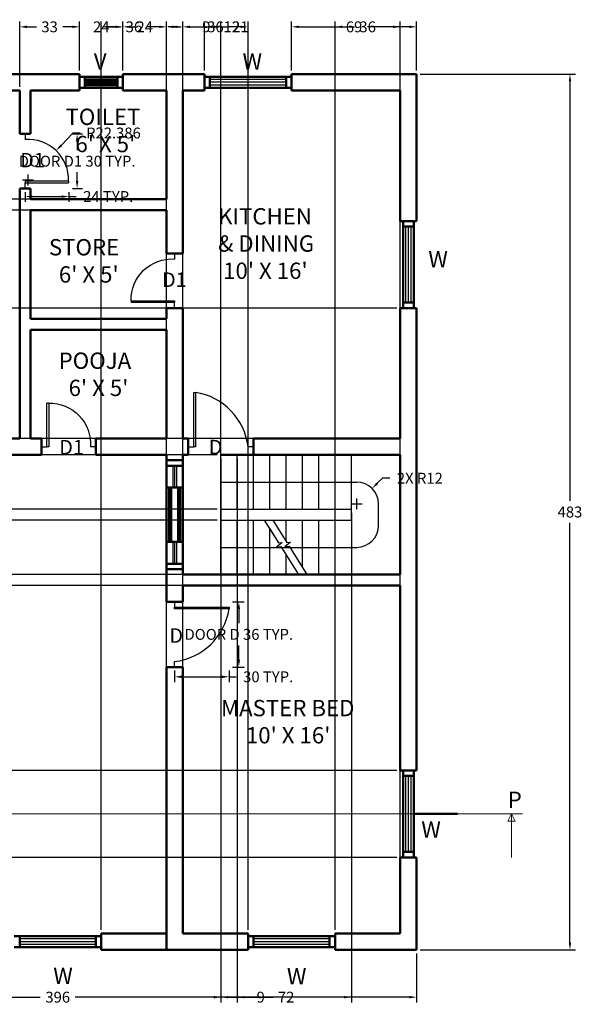
# Model space of a CAD drawing. Units: inches. Extents: x 853 to 2068, y 1026 to 2097.
# Tile 2 of 6: x 1122 to 1432, y 1026 to 1569. Entities that reach past the tile are written whole.
import ezdxf

# ---------------------------------------------------------------- set-up
doc = ezdxf.new("R2010")
doc.units = ezdxf.units.IN
doc.header["$MEASUREMENT"] = 0
for name, color, linetype, lineweight in [('A-ANNO-DIMS', 2, 'Continuous', 18), ('A-ANNO-SYMB', 2, 'Continuous', 18), ('A-ANNO-TEXT', 3, 'Continuous', 18), ('A-AREA-IDEN', 7, 'Continuous', 18), ('A-DOOR', 3, 'Continuous', 25), ('A-FLOR-STRS', 6, 'Continuous', 25), ('A-GLAZ', 4, 'Continuous', 25), ('A-WALL', 7, 'Continuous', 50)]:
    doc.layers.add(name, color=color, linetype=linetype, lineweight=lineweight)
doc.styles.get("Standard").update_dxf_attribs({"font": 'arial.ttf'})
doc.dimstyles.get("Standard").update_dxf_attribs({"dimtxt": 6, "dimasz": 4, "dimexe": 3, "dimexo": 2, "dimgap": 3, "dimtad": 0, "dimtih": 1, "dimtoh": 1, "dimdec": 0, "dimzin": 0, "dimdsep": 46, "dimlunit": 3, "dimtxsty": 'Standard', "dimcen": 3, "dimadec": 0, "dimazin": 0, "dimtfac": 1, "dimtdec": 0, "dimtofl": 0, "dimtmove": 0, "dimatfit": 3, "dimfxl": 1, "dimtolj": 1, "dimtzin": 0, "dimarcsym": 0})

# ---------------------------------------------------------------- blocks, each defined once
blk = doc.blocks.new('DOOR-D')
for p, q in [((0, 36), (0, 33)), ((0, 33), (30, 33)), ((0, 32), (0, 33)), ((30, 33), (30, 32)), ((30, 32), (0, 32)), ((0, 0), (0, 3))]:
    blk.add_line(p, q)
blk.add_arc((-4.1, 37.26), 34.5, 276.8214, 351.2366)
blk = doc.blocks.new('DOOR-D1')
for p, q in [((0, 30), (0, 27)), ((24, 4), (0, 4)), ((0, 4), (0, 3)), ((0, 0), (0, 3)), ((0, 3), (24, 3)), ((24, 4), (24, 3))]:
    blk.add_line(p, q)
blk.add_arc((1.62, 4.67), 22.39, 358.2784, 94.1594)
blk = doc.blocks.new('*D5')
at = {"layer": 'A-ANNO-DIMS', "color": 0, "lineweight": -2, "transparency": 16777216}
for p, q in [((1239.25, 1248.25), (1245.65, 1248.25)), ((1242.65, 1244.25), (1242.65, 1236.36)), ((1242.65, 1216.25), (1242.65, 1224.14)), ((1239.25, 1212.25), (1245.65, 1212.25))]:
    blk.add_line(p, q, dxfattribs=at)
at = {"layer": 'A-ANNO-DIMS', "color": 0, "transparency": 16777216}
for points in [[(1241.98, 1244.25), (1243.32, 1244.25), (1242.65, 1248.25)], [(1241.98, 1216.25), (1243.32, 1216.25), (1242.65, 1212.25)]]:
    blk.add_solid(points, dxfattribs=at)
at = {"layer": 'Defpoints', "color": 0, "transparency": 16777216}
for p in [(1237.25, 1248.25), (1242.65, 1248.25), (1237.25, 1212.25)]:
    blk.add_point(p, dxfattribs=at)
at = {"layer": 'A-ANNO-DIMS', "color": 0, "transparency": 16777216, "insert": (1242.65, 1230.25), "char_height": 6, "attachment_point": 5}
blk.add_mtext('\\A1;DOOR D 36 TYP.', dxfattribs=at)
blk = doc.blocks.new('*D6')
at = {"layer": 'A-ANNO-DIMS', "color": 0, "lineweight": -2, "transparency": 16777216}
for p, q in [((1207.25, 1210.25), (1207.25, 1203.85)), ((1211.25, 1206.85), (1233.25, 1206.85)), ((1237.25, 1210.25), (1237.25, 1203.85)), ((1237.25, 1206.85), (1241.25, 1206.85))]:
    blk.add_line(p, q, dxfattribs=at)
at = {"layer": 'A-ANNO-DIMS', "color": 0, "transparency": 16777216}
for points in [[(1211.25, 1207.52), (1211.25, 1206.18), (1207.25, 1206.85)], [(1233.25, 1207.52), (1233.25, 1206.18), (1237.25, 1206.85)]]:
    blk.add_solid(points, dxfattribs=at)
at = {"layer": 'Defpoints', "color": 0, "transparency": 16777216}
for p in [(1207.25, 1212.25), (1237.25, 1212.25), (1237.25, 1206.85)]:
    blk.add_point(p, dxfattribs=at)
at = {"layer": 'A-ANNO-DIMS', "color": 0, "transparency": 16777216, "insert": (1258.85, 1206.85), "char_height": 6, "attachment_point": 5}
blk.add_mtext('\\A1;30 TYP.', dxfattribs=at)
blk = doc.blocks.new('*D7')
at = {"layer": 'A-ANNO-DIMS', "color": 0, "lineweight": -2, "transparency": 16777216}
for p, q in [((1150.94, 1506.25), (1156.44, 1506.25)), ((1153.44, 1502.25), (1153.44, 1497.36)), ((1153.44, 1480.25), (1153.44, 1485.14)), ((1150.94, 1476.25), (1156.44, 1476.25))]:
    blk.add_line(p, q, dxfattribs=at)
at = {"layer": 'A-ANNO-DIMS', "color": 0, "transparency": 16777216}
for points in [[(1152.77, 1502.25), (1154.11, 1502.25), (1153.44, 1506.25)], [(1152.77, 1480.25), (1154.11, 1480.25), (1153.44, 1476.25)]]:
    blk.add_solid(points, dxfattribs=at)
at = {"layer": 'Defpoints', "color": 0, "transparency": 16777216}
for p in [(1148.94, 1506.25), (1153.44, 1506.25), (1148.94, 1476.25)]:
    blk.add_point(p, dxfattribs=at)
at = {"layer": 'A-ANNO-DIMS', "color": 0, "transparency": 16777216, "insert": (1153.44, 1491.25), "char_height": 6, "attachment_point": 5}
blk.add_mtext('\\A1;DOOR D1 30 TYP.', dxfattribs=at)
blk = doc.blocks.new('*D8')
at = {"layer": 'A-ANNO-DIMS', "color": 0, "lineweight": -2, "transparency": 16777216}
for p, q in [((1124.75, 1474.25), (1124.75, 1468.75)), ((1128.75, 1471.75), (1144.94, 1471.75)), ((1148.94, 1474.25), (1148.94, 1468.75)), ((1148.94, 1471.75), (1152.94, 1471.75))]:
    blk.add_line(p, q, dxfattribs=at)
at = {"layer": 'A-ANNO-DIMS', "color": 0, "transparency": 16777216}
for points in [[(1128.75, 1472.42), (1128.75, 1471.08), (1124.75, 1471.75)], [(1144.94, 1472.42), (1144.94, 1471.08), (1148.94, 1471.75)]]:
    blk.add_solid(points, dxfattribs=at)
at = {"layer": 'Defpoints', "color": 0, "transparency": 16777216}
for p in [(1124.75, 1476.25), (1148.94, 1476.25), (1148.94, 1471.75)]:
    blk.add_point(p, dxfattribs=at)
at = {"layer": 'A-ANNO-DIMS', "color": 0, "transparency": 16777216, "insert": (1170.6, 1471.75), "char_height": 6, "attachment_point": 5}
blk.add_mtext('\\A1;24 TYP.', dxfattribs=at)
blk = doc.blocks.new('*D13')
at = {"layer": 'A-ANNO-DIMS', "color": 0, "lineweight": -2, "transparency": 16777216}
for p, q in [((944.75, 1054.25), (944.75, 1027.15)), ((1340.75, 1054.25), (1340.75, 1027.15)), ((948.75, 1030.15), (1133.13, 1030.15)), ((1336.75, 1030.15), (1152.38, 1030.15))]:
    blk.add_line(p, q, dxfattribs=at)
at = {"layer": 'A-ANNO-DIMS', "color": 0, "transparency": 16777216}
for points in [[(948.75, 1030.82), (948.75, 1029.48), (944.75, 1030.15)], [(1336.75, 1030.82), (1336.75, 1029.48), (1340.75, 1030.15)]]:
    blk.add_solid(points, dxfattribs=at)
at = {"layer": 'Defpoints', "color": 0, "transparency": 16777216}
for p in [(944.75, 1056.25), (1340.75, 1056.25), (1340.75, 1030.15)]:
    blk.add_point(p, dxfattribs=at)
at = {"layer": 'A-ANNO-DIMS', "color": 0, "transparency": 16777216, "insert": (1142.75, 1030.15), "char_height": 6, "attachment_point": 5}
blk.add_mtext('\\A1;396', dxfattribs=at)
blk = doc.blocks.new('*D16')
at = {"layer": 'A-ANNO-DIMS', "color": 0, "lineweight": -2, "transparency": 16777216}
for p, q in [((1166.75, 1067.25), (1166.75, 1568.35)), ((1170.75, 1565.35), (1177.46, 1565.35)), ((1198.75, 1565.35), (1192.04, 1565.35)), ((1202.75, 1067.25), (1202.75, 1568.35))]:
    blk.add_line(p, q, dxfattribs=at)
at = {"layer": 'A-ANNO-DIMS', "color": 0, "transparency": 16777216}
for points in [[(1170.75, 1566.02), (1170.75, 1564.68), (1166.75, 1565.35)], [(1198.75, 1566.02), (1198.75, 1564.68), (1202.75, 1565.35)]]:
    blk.add_solid(points, dxfattribs=at)
at = {"layer": 'Defpoints', "color": 0, "transparency": 16777216}
for p in [(1202.75, 1565.35), (1166.75, 1065.25), (1202.75, 1065.25)]:
    blk.add_point(p, dxfattribs=at)
at = {"layer": 'A-ANNO-DIMS', "color": 0, "transparency": 16777216, "insert": (1184.75, 1565.35), "char_height": 6, "attachment_point": 5}
blk.add_mtext('\\A1;36', dxfattribs=at)
blk = doc.blocks.new('*D17')
at = {"layer": 'A-ANNO-DIMS', "color": 0, "lineweight": -2, "transparency": 16777216}
for p, q in [((1211.75, 1067.25), (1211.75, 1568.35)), ((1215.75, 1565.35), (1222.46, 1565.35)), ((1243.75, 1565.35), (1237.04, 1565.35)), ((1247.75, 1067.25), (1247.75, 1568.35))]:
    blk.add_line(p, q, dxfattribs=at)
at = {"layer": 'A-ANNO-DIMS', "color": 0, "transparency": 16777216}
for points in [[(1215.75, 1566.02), (1215.75, 1564.68), (1211.75, 1565.35)], [(1243.75, 1566.02), (1243.75, 1564.68), (1247.75, 1565.35)]]:
    blk.add_solid(points, dxfattribs=at)
at = {"layer": 'Defpoints', "color": 0, "transparency": 16777216}
for p in [(1247.75, 1565.35), (1211.75, 1065.25), (1247.75, 1065.25)]:
    blk.add_point(p, dxfattribs=at)
at = {"layer": 'A-ANNO-DIMS', "color": 0, "transparency": 16777216, "insert": (1229.75, 1565.35), "char_height": 6, "attachment_point": 5}
blk.add_mtext('\\A1;36', dxfattribs=at)
blk = doc.blocks.new('*D18')
at = {"layer": 'A-ANNO-DIMS', "color": 0, "lineweight": -2, "transparency": 16777216}
for p, q in [((1295.75, 1067.25), (1295.75, 1568.35)), ((1299.75, 1565.35), (1306.46, 1565.35)), ((1327.75, 1565.35), (1321.04, 1565.35)), ((1331.75, 1067.25), (1331.75, 1568.35))]:
    blk.add_line(p, q, dxfattribs=at)
at = {"layer": 'A-ANNO-DIMS', "color": 0, "transparency": 16777216}
for points in [[(1299.75, 1566.02), (1299.75, 1564.68), (1295.75, 1565.35)], [(1327.75, 1566.02), (1327.75, 1564.68), (1331.75, 1565.35)]]:
    blk.add_solid(points, dxfattribs=at)
at = {"layer": 'Defpoints', "color": 0, "transparency": 16777216}
for p in [(1331.75, 1565.35), (1295.75, 1065.25), (1331.75, 1065.25)]:
    blk.add_point(p, dxfattribs=at)
at = {"layer": 'A-ANNO-DIMS', "color": 0, "transparency": 16777216, "insert": (1313.75, 1565.35), "char_height": 6, "attachment_point": 5}
blk.add_mtext('\\A1;36', dxfattribs=at)
blk = doc.blocks.new('*D22')
at = {"layer": 'A-ANNO-DIMS', "color": 0, "lineweight": -2, "transparency": 16777216}
for p, q in [((1121.75, 1532.25), (1121.75, 1568.35)), ((1125.75, 1565.35), (1130.96, 1565.35)), ((1150.75, 1565.35), (1145.55, 1565.35)), ((1154.75, 1541.25), (1154.75, 1568.35))]:
    blk.add_line(p, q, dxfattribs=at)
at = {"layer": 'A-ANNO-DIMS', "color": 0, "transparency": 16777216}
for points in [[(1125.75, 1566.02), (1125.75, 1564.68), (1121.75, 1565.35)], [(1150.75, 1566.02), (1150.75, 1564.68), (1154.75, 1565.35)]]:
    blk.add_solid(points, dxfattribs=at)
at = {"layer": 'Defpoints', "color": 0, "transparency": 16777216}
for p in [(1154.75, 1565.35), (1154.75, 1539.25), (1121.75, 1530.25)]:
    blk.add_point(p, dxfattribs=at)
at = {"layer": 'A-ANNO-DIMS', "color": 0, "transparency": 16777216, "insert": (1138.25, 1565.35), "char_height": 6, "attachment_point": 5}
blk.add_mtext('\\A1;33', dxfattribs=at)
blk = doc.blocks.new('*D23')
at = {"layer": 'A-ANNO-DIMS', "color": 0, "lineweight": -2, "transparency": 16777216}
for p, q in [((1150.75, 1565.35), (1146.75, 1565.35)), ((1154.75, 1541.25), (1154.75, 1568.35)), ((1178.75, 1541.25), (1178.75, 1568.35)), ((1182.75, 1565.35), (1186.75, 1565.35))]:
    blk.add_line(p, q, dxfattribs=at)
at = {"layer": 'A-ANNO-DIMS', "color": 0, "transparency": 16777216}
for points in [[(1150.75, 1566.02), (1150.75, 1564.68), (1154.75, 1565.35)], [(1182.75, 1566.02), (1182.75, 1564.68), (1178.75, 1565.35)]]:
    blk.add_solid(points, dxfattribs=at)
at = {"layer": 'Defpoints', "color": 0, "transparency": 16777216}
for p in [(1178.75, 1565.35), (1154.75, 1539.25), (1178.75, 1539.25)]:
    blk.add_point(p, dxfattribs=at)
at = {"layer": 'A-ANNO-DIMS', "color": 0, "transparency": 16777216, "insert": (1166.75, 1565.35), "char_height": 6, "attachment_point": 5}
blk.add_mtext('\\A1;24', dxfattribs=at)
blk = doc.blocks.new('*D24')
at = {"layer": 'A-ANNO-DIMS', "color": 0, "lineweight": -2, "transparency": 16777216}
for p, q in [((1174.75, 1565.35), (1170.75, 1565.35)), ((1178.75, 1541.25), (1178.75, 1568.35)), ((1202.75, 1532.25), (1202.75, 1568.35)), ((1206.75, 1565.35), (1210.75, 1565.35))]:
    blk.add_line(p, q, dxfattribs=at)
at = {"layer": 'A-ANNO-DIMS', "color": 0, "transparency": 16777216}
for points in [[(1174.75, 1566.02), (1174.75, 1564.68), (1178.75, 1565.35)], [(1206.75, 1566.02), (1206.75, 1564.68), (1202.75, 1565.35)]]:
    blk.add_solid(points, dxfattribs=at)
at = {"layer": 'Defpoints', "color": 0, "transparency": 16777216}
for p in [(1202.75, 1565.35), (1178.75, 1539.25), (1202.75, 1530.25)]:
    blk.add_point(p, dxfattribs=at)
at = {"layer": 'A-ANNO-DIMS', "color": 0, "transparency": 16777216, "insert": (1190.75, 1565.35), "char_height": 6, "attachment_point": 5}
blk.add_mtext('\\A1;24', dxfattribs=at)
blk = doc.blocks.new('*D25')
at = {"layer": 'A-ANNO-DIMS', "color": 0, "lineweight": -2, "transparency": 16777216}
for p, q in [((1198.75, 1565.35), (1194.75, 1565.35)), ((1202.75, 1532.25), (1202.75, 1568.35)), ((1211.75, 1532.25), (1211.75, 1568.35)), ((1215.75, 1565.35), (1219.75, 1565.35))]:
    blk.add_line(p, q, dxfattribs=at)
at = {"layer": 'A-ANNO-DIMS', "color": 0, "transparency": 16777216}
for points in [[(1198.75, 1566.02), (1198.75, 1564.68), (1202.75, 1565.35)], [(1215.75, 1566.02), (1215.75, 1564.68), (1211.75, 1565.35)]]:
    blk.add_solid(points, dxfattribs=at)
at = {"layer": 'Defpoints', "color": 0, "transparency": 16777216}
for p in [(1211.75, 1565.35), (1202.75, 1530.25), (1211.75, 1530.25)]:
    blk.add_point(p, dxfattribs=at)
at = {"layer": 'A-ANNO-DIMS', "color": 0, "transparency": 16777216, "insert": (1224.72, 1565.35), "char_height": 6, "attachment_point": 5}
blk.add_mtext('\\A1;9', dxfattribs=at)
blk = doc.blocks.new('*D26')
at = {"layer": 'A-ANNO-DIMS', "color": 0, "lineweight": -2, "transparency": 16777216}
for p, q in [((1207.75, 1565.35), (1203.75, 1565.35)), ((1211.75, 1532.25), (1211.75, 1568.35)), ((1223.75, 1541.25), (1223.75, 1568.35)), ((1227.75, 1565.35), (1231.75, 1565.35))]:
    blk.add_line(p, q, dxfattribs=at)
at = {"layer": 'A-ANNO-DIMS', "color": 0, "transparency": 16777216}
for points in [[(1207.75, 1566.02), (1207.75, 1564.68), (1211.75, 1565.35)], [(1227.75, 1566.02), (1227.75, 1564.68), (1223.75, 1565.35)]]:
    blk.add_solid(points, dxfattribs=at)
at = {"layer": 'Defpoints', "color": 0, "transparency": 16777216}
for p in [(1223.75, 1565.35), (1223.75, 1539.25), (1211.75, 1530.25)]:
    blk.add_point(p, dxfattribs=at)
at = {"layer": 'A-ANNO-DIMS', "color": 0, "transparency": 16777216, "insert": (1238.74, 1565.35), "char_height": 6, "attachment_point": 5}
blk.add_mtext('\\A1;12', dxfattribs=at)
blk = doc.blocks.new('*D27')
at = {"layer": 'A-ANNO-DIMS', "color": 0, "lineweight": -2, "transparency": 16777216}
for p, q in [((1271.75, 1541.25), (1271.75, 1568.35)), ((1275.75, 1565.35), (1298.93, 1565.35)), ((1336.75, 1565.35), (1313.57, 1565.35)), ((1340.75, 1541.25), (1340.75, 1568.35))]:
    blk.add_line(p, q, dxfattribs=at)
at = {"layer": 'A-ANNO-DIMS', "color": 0, "transparency": 16777216}
for points in [[(1275.75, 1566.02), (1275.75, 1564.68), (1271.75, 1565.35)], [(1336.75, 1566.02), (1336.75, 1564.68), (1340.75, 1565.35)]]:
    blk.add_solid(points, dxfattribs=at)
at = {"layer": 'Defpoints', "color": 0, "transparency": 16777216}
for p in [(1340.75, 1565.35), (1271.75, 1539.25), (1340.75, 1539.25)]:
    blk.add_point(p, dxfattribs=at)
at = {"layer": 'A-ANNO-DIMS', "color": 0, "transparency": 16777216, "insert": (1306.25, 1565.35), "char_height": 6, "attachment_point": 5}
blk.add_mtext('\\A1;69', dxfattribs=at)
blk = doc.blocks.new('*D34')
at = {"layer": 'A-ANNO-DIMS', "color": 0, "lineweight": -2, "transparency": 16777216}
for p, q in [((1342.75, 1539.25), (1428.35, 1539.25)), ((1425.35, 1535.25), (1425.35, 1303.82)), ((1425.35, 1060.25), (1425.35, 1291.69)), ((1342.75, 1056.25), (1428.35, 1056.25))]:
    blk.add_line(p, q, dxfattribs=at)
at = {"layer": 'A-ANNO-DIMS', "color": 0, "transparency": 16777216}
for points in [[(1424.68, 1535.25), (1426.02, 1535.25), (1425.35, 1539.25)], [(1424.68, 1060.25), (1426.02, 1060.25), (1425.35, 1056.25)]]:
    blk.add_solid(points, dxfattribs=at)
at = {"layer": 'Defpoints', "color": 0, "transparency": 16777216}
for p in [(1340.75, 1539.25), (1425.35, 1539.25), (1340.75, 1056.25)]:
    blk.add_point(p, dxfattribs=at)
at = {"layer": 'A-ANNO-DIMS', "color": 0, "transparency": 16777216, "insert": (1425.35, 1297.75), "char_height": 6, "attachment_point": 5}
blk.add_mtext('\\A1;483', dxfattribs=at)
blk = doc.blocks.new('*D35')
at = {"layer": 'A-ANNO-DIMS', "color": 0, "lineweight": -2, "transparency": 16777216}
for p, q in [((1329.75, 1155.25), (857.15, 1155.25)), ((860.15, 1151.25), (860.15, 1137.31)), ((860.15, 1111.25), (860.15, 1125.19)), ((1329.75, 1107.25), (857.15, 1107.25))]:
    blk.add_line(p, q, dxfattribs=at)
at = {"layer": 'A-ANNO-DIMS', "color": 0, "transparency": 16777216}
for points in [[(859.48, 1151.25), (860.82, 1151.25), (860.15, 1155.25)], [(859.48, 1111.25), (860.82, 1111.25), (860.15, 1107.25)]]:
    blk.add_solid(points, dxfattribs=at)
at = {"layer": 'Defpoints', "color": 0, "transparency": 16777216}
for p in [(860.15, 1155.25), (1331.75, 1155.25), (1331.75, 1107.25)]:
    blk.add_point(p, dxfattribs=at)
at = {"layer": 'A-ANNO-DIMS', "color": 0, "transparency": 16777216, "insert": (860.15, 1131.25), "char_height": 6, "attachment_point": 5}
blk.add_mtext('\\A1;48', dxfattribs=at)
blk = doc.blocks.new('*D36')
at = {"layer": 'A-ANNO-DIMS', "color": 0, "lineweight": -2, "transparency": 16777216}
for p, q in [((1329.75, 1257.25), (857.15, 1257.25)), ((860.15, 1253.25), (860.15, 1212.31)), ((860.15, 1159.25), (860.15, 1200.19)), ((1329.75, 1155.25), (857.15, 1155.25))]:
    blk.add_line(p, q, dxfattribs=at)
at = {"layer": 'A-ANNO-DIMS', "color": 0, "transparency": 16777216}
for points in [[(859.48, 1253.25), (860.82, 1253.25), (860.15, 1257.25)], [(859.48, 1159.25), (860.82, 1159.25), (860.15, 1155.25)]]:
    blk.add_solid(points, dxfattribs=at)
at = {"layer": 'Defpoints', "color": 0, "transparency": 16777216}
for p in [(860.15, 1257.25), (1331.75, 1257.25), (1331.75, 1155.25)]:
    blk.add_point(p, dxfattribs=at)
at = {"layer": 'A-ANNO-DIMS', "color": 0, "transparency": 16777216, "insert": (860.15, 1206.25), "char_height": 6, "attachment_point": 5}
blk.add_mtext('\\A1;102', dxfattribs=at)
blk = doc.blocks.new('*D37')
at = {"layer": 'A-ANNO-DIMS', "color": 0, "lineweight": -2, "transparency": 16777216}
for p, q in [((860.15, 1267.25), (860.15, 1271.25)), ((860.15, 1271.25), (864.15, 1271.25)), ((1329.75, 1263.25), (857.15, 1263.25)), ((1329.75, 1257.25), (857.15, 1257.25)), ((860.15, 1253.25), (860.15, 1249.25))]:
    blk.add_line(p, q, dxfattribs=at)
at = {"layer": 'A-ANNO-DIMS', "color": 0, "transparency": 16777216}
for points in [[(859.48, 1267.25), (860.82, 1267.25), (860.15, 1263.25)], [(859.48, 1253.25), (860.82, 1253.25), (860.15, 1257.25)]]:
    blk.add_solid(points, dxfattribs=at)
at = {"layer": 'Defpoints', "color": 0, "transparency": 16777216}
for p in [(860.15, 1263.25), (1331.75, 1263.25), (1331.75, 1257.25)]:
    blk.add_point(p, dxfattribs=at)
at = {"layer": 'A-ANNO-DIMS', "color": 0, "transparency": 16777216, "insert": (869.13, 1271.25), "char_height": 6, "attachment_point": 5}
blk.add_mtext('\\A1;6', dxfattribs=at)
blk = doc.blocks.new('*D38')
at = {"layer": 'A-ANNO-DIMS', "color": 0, "lineweight": -2, "transparency": 16777216}
for p, q in [((1329.75, 1410.25), (857.15, 1410.25)), ((860.15, 1406.25), (860.15, 1380.26)), ((860.15, 1342.25), (860.15, 1368.24)), ((1329.75, 1338.25), (857.15, 1338.25))]:
    blk.add_line(p, q, dxfattribs=at)
at = {"layer": 'A-ANNO-DIMS', "color": 0, "transparency": 16777216}
for points in [[(859.48, 1406.25), (860.82, 1406.25), (860.15, 1410.25)], [(859.48, 1342.25), (860.82, 1342.25), (860.15, 1338.25)]]:
    blk.add_solid(points, dxfattribs=at)
at = {"layer": 'Defpoints', "color": 0, "transparency": 16777216}
for p in [(860.15, 1410.25), (1331.75, 1410.25), (1331.75, 1338.25)]:
    blk.add_point(p, dxfattribs=at)
at = {"layer": 'A-ANNO-DIMS', "color": 0, "transparency": 16777216, "insert": (860.15, 1374.25), "char_height": 6, "attachment_point": 5}
blk.add_mtext('\\A1;72', dxfattribs=at)
blk = doc.blocks.new('*D39')
at = {"layer": 'A-ANNO-DIMS', "color": 0, "lineweight": -2, "transparency": 16777216}
for p, q in [((860.15, 1474.25), (860.15, 1478.25)), ((860.15, 1478.25), (864.15, 1478.25)), ((1200.75, 1470.25), (857.15, 1470.25)), ((1200.75, 1464.25), (857.15, 1464.25)), ((860.15, 1460.25), (860.15, 1456.25))]:
    blk.add_line(p, q, dxfattribs=at)
at = {"layer": 'A-ANNO-DIMS', "color": 0, "transparency": 16777216}
for points in [[(859.48, 1474.25), (860.82, 1474.25), (860.15, 1470.25)], [(859.48, 1460.25), (860.82, 1460.25), (860.15, 1464.25)]]:
    blk.add_solid(points, dxfattribs=at)
at = {"layer": 'Defpoints', "color": 0, "transparency": 16777216}
for p in [(860.15, 1470.25), (1202.75, 1470.25), (1202.75, 1464.25)]:
    blk.add_point(p, dxfattribs=at)
at = {"layer": 'A-ANNO-DIMS', "color": 0, "transparency": 16777216, "insert": (869.13, 1478.25), "char_height": 6, "attachment_point": 5}
blk.add_mtext('\\A1;6', dxfattribs=at)
blk = doc.blocks.new('*D40')
at = {"layer": 'A-ANNO-DIMS', "color": 0, "lineweight": -2, "transparency": 16777216}
for p, q in [((1211.75, 1265.25), (1211.75, 1568.35)), ((1215.75, 1565.35), (1228.75, 1565.35)), ((1232.75, 1265.25), (1232.75, 1568.35)), ((1232.75, 1565.35), (1236.75, 1565.35))]:
    blk.add_line(p, q, dxfattribs=at)
at = {"layer": 'A-ANNO-DIMS', "color": 0, "transparency": 16777216}
for points in [[(1215.75, 1566.02), (1215.75, 1564.68), (1211.75, 1565.35)], [(1228.75, 1566.02), (1228.75, 1564.68), (1232.75, 1565.35)]]:
    blk.add_solid(points, dxfattribs=at)
at = {"layer": 'Defpoints', "color": 0, "transparency": 16777216}
for p in [(1232.75, 1565.35), (1211.75, 1263.25), (1232.75, 1263.25)]:
    blk.add_point(p, dxfattribs=at)
at = {"layer": 'A-ANNO-DIMS', "color": 0, "transparency": 16777216, "insert": (1243.52, 1565.35), "char_height": 6, "attachment_point": 5}
blk.add_mtext('\\A1;21', dxfattribs=at)
blk = doc.blocks.new('*D41')
at = {"layer": 'A-ANNO-DIMS', "color": 0, "lineweight": -2, "transparency": 16777216}
for p, q in [((1232.75, 1327.25), (1232.75, 1027.15)), ((1241.75, 1327.25), (1241.75, 1027.15)), ((1228.75, 1030.15), (1224.75, 1030.15)), ((1245.75, 1030.15), (1249.75, 1030.15))]:
    blk.add_line(p, q, dxfattribs=at)
at = {"layer": 'A-ANNO-DIMS', "color": 0, "transparency": 16777216}
for points in [[(1228.75, 1030.82), (1228.75, 1029.48), (1232.75, 1030.15)], [(1245.75, 1030.82), (1245.75, 1029.48), (1241.75, 1030.15)]]:
    blk.add_solid(points, dxfattribs=at)
at = {"layer": 'Defpoints', "color": 0, "transparency": 16777216}
for p in [(1232.75, 1329.25), (1241.75, 1329.25), (1241.75, 1030.15)]:
    blk.add_point(p, dxfattribs=at)
at = {"layer": 'A-ANNO-DIMS', "color": 0, "transparency": 16777216, "insert": (1254.72, 1030.15), "char_height": 6, "attachment_point": 5}
blk.add_mtext('\\A1;9', dxfattribs=at)
blk = doc.blocks.new('*D42')
at = {"layer": 'A-ANNO-DIMS', "color": 0, "lineweight": -2, "transparency": 16777216}
for p, q in [((1232.75, 1297.25), (1232.75, 1027.15)), ((1304.75, 1297.25), (1304.75, 1027.15)), ((1236.75, 1030.15), (1261.51, 1030.15)), ((1300.75, 1030.15), (1275.99, 1030.15))]:
    blk.add_line(p, q, dxfattribs=at)
at = {"layer": 'A-ANNO-DIMS', "color": 0, "transparency": 16777216}
for points in [[(1236.75, 1030.82), (1236.75, 1029.48), (1232.75, 1030.15)], [(1300.75, 1030.82), (1300.75, 1029.48), (1304.75, 1030.15)]]:
    blk.add_solid(points, dxfattribs=at)
at = {"layer": 'Defpoints', "color": 0, "transparency": 16777216}
for p in [(1232.75, 1299.25), (1304.75, 1299.25), (1304.75, 1030.15)]:
    blk.add_point(p, dxfattribs=at)
at = {"layer": 'A-ANNO-DIMS', "color": 0, "transparency": 16777216, "insert": (1268.75, 1030.15), "char_height": 6, "attachment_point": 5}
blk.add_mtext('\\A1;72', dxfattribs=at)
blk = doc.blocks.new('*D43')
at = {"layer": 'A-ANNO-DIMS', "color": 0, "lineweight": -2, "transparency": 16777216}
for p, q in [((1230.75, 1293.25), (857.15, 1293.25)), ((860.15, 1289.25), (860.15, 1284.32)), ((860.15, 1267.25), (860.15, 1272.19)), ((1230.75, 1263.25), (857.15, 1263.25))]:
    blk.add_line(p, q, dxfattribs=at)
at = {"layer": 'A-ANNO-DIMS', "color": 0, "transparency": 16777216}
for points in [[(859.48, 1289.25), (860.82, 1289.25), (860.15, 1293.25)], [(859.48, 1267.25), (860.82, 1267.25), (860.15, 1263.25)]]:
    blk.add_solid(points, dxfattribs=at)
at = {"layer": 'Defpoints', "color": 0, "transparency": 16777216}
for p in [(860.15, 1293.25), (1232.75, 1293.25), (1232.75, 1263.25)]:
    blk.add_point(p, dxfattribs=at)
at = {"layer": 'A-ANNO-DIMS', "color": 0, "transparency": 16777216, "insert": (860.15, 1278.25), "char_height": 6, "attachment_point": 5}
blk.add_mtext('\\A1;30', dxfattribs=at)
blk = doc.blocks.new('*D44')
at = {"layer": 'A-ANNO-DIMS', "color": 0, "lineweight": -2, "transparency": 16777216}
for p, q in [((1230.75, 1329.25), (857.15, 1329.25)), ((860.15, 1325.25), (860.15, 1320.32)), ((860.15, 1303.25), (860.15, 1308.19)), ((1230.75, 1299.25), (857.15, 1299.25))]:
    blk.add_line(p, q, dxfattribs=at)
at = {"layer": 'A-ANNO-DIMS', "color": 0, "transparency": 16777216}
for points in [[(859.48, 1325.25), (860.82, 1325.25), (860.15, 1329.25)], [(859.48, 1303.25), (860.82, 1303.25), (860.15, 1299.25)]]:
    blk.add_solid(points, dxfattribs=at)
at = {"layer": 'Defpoints', "color": 0, "transparency": 16777216}
for p in [(860.15, 1329.25), (1232.75, 1329.25), (1232.75, 1299.25)]:
    blk.add_point(p, dxfattribs=at)
at = {"layer": 'A-ANNO-DIMS', "color": 0, "transparency": 16777216, "insert": (860.15, 1314.25), "char_height": 6, "attachment_point": 5}
blk.add_mtext('\\A1;30', dxfattribs=at)
blk = doc.blocks.new('*D116')
at = {"layer": 'A-ANNO-DIMS', "color": 0, "lineweight": -2, "transparency": 16777216}
for p, q in [((1151.16, 1506.78), (1144.63, 1499.97)), ((1155.16, 1506.78), (1151.16, 1506.78)), ((1126.37, 1477.92), (1126.37, 1483.92)), ((1123.37, 1480.92), (1129.37, 1480.92))]:
    blk.add_line(p, q, dxfattribs=at)
at = {"layer": 'A-ANNO-DIMS', "color": 0, "transparency": 16777216}
blk.add_solid([(1144.15, 1500.44), (1145.11, 1499.51), (1141.86, 1497.09)], dxfattribs=at)
at = {"layer": 'Defpoints', "color": 0, "transparency": 16777216}
for p in [(1141.86, 1497.09), (1126.37, 1480.92)]:
    blk.add_point(p, dxfattribs=at)
at = {"layer": 'A-ANNO-DIMS', "color": 0, "transparency": 16777216, "insert": (1173.48, 1506.78), "char_height": 6, "attachment_point": 5}
blk.add_mtext('\\A1;R22.386', dxfattribs=at)
blk = doc.blocks.new('*D117')
at = {"layer": 'A-ANNO-DIMS', "color": 0, "lineweight": -2, "transparency": 16777216}
for p, q in [((1321.89, 1316.39), (1319.06, 1313.57)), ((1325.89, 1316.39), (1321.89, 1316.39)), ((1307.75, 1299.25), (1307.75, 1305.25)), ((1304.75, 1302.25), (1310.75, 1302.25))]:
    blk.add_line(p, q, dxfattribs=at)
at = {"layer": 'A-ANNO-DIMS', "color": 0, "transparency": 16777216}
blk.add_solid([(1318.59, 1314.04), (1319.54, 1313.09), (1316.24, 1310.74)], dxfattribs=at)
at = {"layer": 'Defpoints', "color": 0, "transparency": 16777216}
for p in [(1316.24, 1310.74), (1307.75, 1302.25)]:
    blk.add_point(p, dxfattribs=at)
at = {"layer": 'A-ANNO-DIMS', "color": 0, "transparency": 16777216, "insert": (1342.53, 1316.39), "char_height": 6, "attachment_point": 5}
blk.add_mtext('\\A1;2X R12', dxfattribs=at)

msp = doc.modelspace()

# ---------------------------------------------------------------- linework, layer by layer
at = {"layer": 'A-ANNO-SYMB'}
for p, q in [((886.251, 1131.2513), (1399.251, 1131.2513)), ((1391.1127, 1127.2513), (1393.1127, 1131.2513)), ((1393.1127, 1131.2513), (1393.1127, 1107.2513)), ((1393.1127, 1131.2513), (1393.1127, 1127.2513)), ((1395.1127, 1127.2513), (1393.1127, 1131.2513)), ((1393.1127, 1131.2513), (1393.1127, 1127.2513)), ((1393.1127, 1127.2513), (1391.1127, 1127.2513)), ((1393.1127, 1127.2513), (1395.1127, 1127.2513))]:
    msp.add_line(p, q, dxfattribs=at)
at = {"layer": 'A-FLOR-STRS'}
for p, q in [((1232.751, 1299.2513), (1232.751, 1329.2513)), ((1241.751, 1299.2513), (1241.751, 1329.2513)), ((1250.751, 1299.2513), (1250.751, 1329.2513)), ((1259.751, 1299.2513), (1259.751, 1329.2513)), ((1268.751, 1299.2513), (1268.751, 1329.2513)), ((1277.751, 1299.2513), (1277.751, 1329.2513)), ((1286.751, 1299.2513), (1286.751, 1329.2513)), ((1295.751, 1299.2513), (1295.751, 1329.2513)), ((1304.751, 1293.2513), (1304.751, 1329.2513)), ((1232.751, 1314.2513), (1307.751, 1314.2513)), ((1232.751, 1299.2513), (1304.751, 1299.2513)), ((1319.751, 1290.2513), (1319.751, 1302.2513)), ((1232.751, 1263.2513), (1232.751, 1293.2513)), ((1232.751, 1293.2513), (1304.751, 1293.2513)), ((1241.751, 1263.2513), (1241.751, 1293.2513)), ((1250.751, 1263.2513), (1250.751, 1293.2513)), ((1256.701, 1293.2513), (1264.5192, 1280.7803)), ((1261.422, 1293.2513), (1268.751, 1281.5607)), ((1268.751, 1281.5607), (1268.751, 1293.2513)), ((1277.751, 1267.2046), (1277.751, 1293.2513)), ((1286.751, 1263.2513), (1286.751, 1293.2513)), ((1295.751, 1263.2513), (1295.751, 1293.2513)), ((1259.751, 1263.2513), (1259.751, 1288.3861)), ((1259.751, 1288.3861), (1264.5192, 1280.7803)), ((1232.751, 1278.2513), (1307.751, 1278.2513)), ((1266.5123, 1280.9455), (1263.4954, 1278.3191)), ((1263.4954, 1278.3191), (1265.8105, 1278.7204)), ((1264.5192, 1280.7803), (1266.5123, 1280.9455)), ((1265.8105, 1278.7204), (1275.5083, 1263.2513)), ((1271.1137, 1281.1363), (1268.0968, 1278.5099)), ((1268.0968, 1278.5099), (1270.412, 1278.9112)), ((1268.751, 1281.5607), (1269.1206, 1280.9712)), ((1269.1206, 1280.9712), (1271.1137, 1281.1363)), ((1270.412, 1278.9112), (1280.2294, 1263.2513)), ((1268.751, 1263.2513), (1268.751, 1274.03))]:
    msp.add_line(p, q, dxfattribs=at)
for centre, start, end in [((1307.751, 1302.2513), 0, 90), ((1307.751, 1290.2513), 270, 0)]:
    msp.add_arc(centre, 12, start, end, dxfattribs=at)
at = {"layer": 'A-GLAZ'}
for p, q in [((1175.751, 1535.7513), (1157.751, 1535.7513)), ((1175.751, 1535.2513), (1157.751, 1535.2513)), ((1175.751, 1534.2513), (1157.751, 1534.2513)), ((1175.751, 1533.7513), (1157.751, 1533.7513)), ((1268.751, 1536.2513), (1226.751, 1536.2513)), ((1268.751, 1534.7513), (1226.751, 1534.7513)), ((1268.751, 1533.2513), (1226.751, 1533.2513)), ((1334.751, 1413.2513), (1334.751, 1455.2513)), ((1336.251, 1413.2513), (1336.251, 1455.2513)), ((1337.751, 1413.2513), (1337.751, 1455.2513)), ((1206.251, 1323.2513), (1206.251, 1311.2513)), ((1207.251, 1323.2513), (1207.251, 1311.2513)), ((1208.251, 1323.2513), (1208.251, 1311.2513)), ((1206.251, 1281.2513), (1206.251, 1269.2513)), ((1207.251, 1281.2513), (1207.251, 1269.2513)), ((1208.251, 1281.2513), (1208.251, 1269.2513)), ((1334.751, 1110.2513), (1334.751, 1152.2513)), ((1336.251, 1110.2513), (1336.251, 1152.2513)), ((1337.751, 1110.2513), (1337.751, 1152.2513)), ((1163.751, 1062.2513), (1121.751, 1062.2513)), ((1163.751, 1060.7513), (1121.751, 1060.7513)), ((1163.751, 1059.2513), (1121.751, 1059.2513)), ((1292.751, 1062.2513), (1250.751, 1062.2513)), ((1292.751, 1060.7513), (1250.751, 1060.7513)), ((1292.751, 1059.2513), (1250.751, 1059.2513))]:
    msp.add_line(p, q, dxfattribs=at)
at = {"layer": 'A-WALL'}
for p, q in [((1061.751, 1539.2513), (1154.751, 1539.2513)), ((1154.751, 1539.2513), (1154.751, 1530.2513)), ((1166.751, 1537.7513), (1154.751, 1537.7513)), ((1157.751, 1537.7513), (1157.751, 1531.7513)), ((1178.751, 1537.7513), (1166.751, 1537.7513)), ((1175.751, 1537.7513), (1175.751, 1531.7513)), ((1178.751, 1539.2513), (1178.751, 1530.2513)), ((1178.751, 1539.2513), (1223.751, 1539.2513)), ((1223.751, 1539.2513), (1223.751, 1530.2513)), ((1271.751, 1537.7513), (1223.751, 1537.7513)), ((1226.751, 1537.7513), (1226.751, 1531.7513)), ((1268.751, 1537.7513), (1268.751, 1531.7513)), ((1271.751, 1539.2513), (1271.751, 1530.2513)), ((1271.751, 1539.2513), (1340.751, 1539.2513)), ((1340.751, 1458.2513), (1340.751, 1539.2513)), ((1166.751, 1531.7513), (1154.751, 1531.7513)), ((1166.751, 1536.2513), (1157.751, 1536.2513)), ((1166.751, 1534.7513), (1157.751, 1534.7513)), ((1166.751, 1533.2513), (1157.751, 1533.2513)), ((1175.751, 1536.2513), (1166.751, 1536.2513)), ((1175.751, 1534.7513), (1166.751, 1534.7513)), ((1175.751, 1533.2513), (1166.751, 1533.2513)), ((1178.751, 1531.7513), (1166.751, 1531.7513)), ((1271.751, 1531.7513), (1223.751, 1531.7513)), ((1061.751, 1530.2513), (1121.751, 1530.2513)), ((1061.751, 1530.2513), (1121.751, 1530.2513)), ((1121.751, 1530.2513), (1121.751, 1506.2513)), ((1127.751, 1530.2513), (1127.751, 1506.2513)), ((1127.751, 1530.2513), (1154.751, 1530.2513)), ((1154.751, 1530.2513), (1130.751, 1530.2513)), ((1202.751, 1530.2513), (1178.751, 1530.2513)), ((1178.751, 1530.2513), (1202.751, 1530.2513)), ((1202.751, 1470.2513), (1202.751, 1530.2513)), ((1211.751, 1530.2513), (1211.751, 1440.2513)), ((1211.751, 1530.2513), (1223.751, 1530.2513)), ((1223.751, 1530.2513), (1211.751, 1530.2513)), ((1331.751, 1530.2513), (1271.751, 1530.2513)), ((1271.751, 1530.2513), (1331.751, 1530.2513)), ((1331.751, 1458.2513), (1331.751, 1530.2513)), ((1331.751, 1458.2513), (1331.751, 1530.2513)), ((1127.751, 1506.2513), (1121.751, 1506.2513)), ((1127.751, 1476.2513), (1121.751, 1476.2513)), ((1121.751, 1476.2513), (1121.751, 1338.2513)), ((1127.751, 1476.2513), (1127.751, 1470.2513)), ((1127.751, 1470.2513), (1202.751, 1470.2513)), ((1127.751, 1464.2513), (1202.751, 1464.2513)), ((1127.751, 1464.2513), (1127.751, 1404.2513)), ((1202.751, 1464.2513), (1202.751, 1440.2513)), ((1340.751, 1458.2513), (1331.751, 1458.2513)), ((1333.251, 1410.2513), (1333.251, 1458.2513)), ((1339.251, 1410.2513), (1339.251, 1458.2513)), ((1339.251, 1455.2513), (1333.251, 1455.2513)), ((1202.751, 1440.2513), (1211.751, 1440.2513)), ((1339.251, 1413.2513), (1333.251, 1413.2513)), ((1202.751, 1410.2513), (1211.751, 1410.2513)), ((1202.751, 1410.2513), (1202.751, 1404.2513)), ((1211.751, 1410.2513), (1211.751, 1338.2513)), ((1331.751, 1338.2513), (1331.751, 1410.2513)), ((1331.751, 1338.2513), (1331.751, 1410.2513)), ((1340.751, 1410.2513), (1331.751, 1410.2513)), ((1340.751, 1155.2513), (1340.751, 1410.2513)), ((1202.751, 1404.2513), (1127.751, 1404.2513)), ((1202.751, 1398.2513), (1127.751, 1398.2513)), ((1127.751, 1398.2513), (1127.751, 1338.2513)), ((1202.751, 1338.2513), (1202.751, 1398.2513)), ((1121.751, 1338.2513), (998.751, 1338.2513)), ((1127.751, 1338.2513), (1133.751, 1338.2513)), ((1127.751, 1338.2513), (1133.751, 1338.2513)), ((1133.751, 1338.2513), (1133.751, 1329.2513)), ((1163.751, 1338.2513), (1163.751, 1329.2513)), ((1163.751, 1338.2513), (1202.751, 1338.2513)), ((1211.751, 1338.2513), (1214.751, 1338.2513)), ((1214.751, 1338.2513), (1214.751, 1329.2513)), ((1250.751, 1338.2513), (1250.751, 1329.2513)), ((1250.751, 1338.2513), (1331.751, 1338.2513)), ((1133.751, 1329.2513), (998.751, 1329.2513)), ((1202.751, 1329.2513), (1163.751, 1329.2513)), ((1202.751, 1248.2513), (1202.751, 1329.2513)), ((1202.751, 1326.2513), (1211.751, 1326.2513)), ((1211.751, 1329.2513), (1214.751, 1329.2513)), ((1211.751, 1329.2513), (1211.751, 1263.2513)), ((1232.751, 1329.2513), (1331.751, 1329.2513)), ((1331.751, 1263.2513), (1331.751, 1329.2513)), ((1202.751, 1323.2513), (1211.751, 1323.2513)), ((1202.751, 1311.2513), (1211.751, 1311.2513)), ((1204.251, 1311.2513), (1204.251, 1281.2513)), ((1205.251, 1311.2513), (1205.251, 1281.2513)), ((1209.251, 1311.2513), (1209.251, 1281.2513)), ((1210.251, 1311.2513), (1210.251, 1281.2513)), ((1211.751, 1281.2513), (1202.751, 1281.2513)), ((1211.751, 1269.2513), (1202.751, 1269.2513)), ((1211.751, 1266.2513), (1202.751, 1266.2513)), ((1211.751, 1263.2513), (1331.751, 1263.2513)), ((1211.751, 1257.2513), (1331.751, 1257.2513)), ((1211.751, 1248.2513), (1211.751, 1257.2513)), ((1331.751, 1257.2513), (1331.751, 1155.2513)), ((1331.751, 1155.2513), (1331.751, 1257.2513)), ((1211.751, 1248.2513), (1202.751, 1248.2513)), ((1202.751, 1065.2513), (1202.751, 1212.2513)), ((1211.751, 1212.2513), (1202.751, 1212.2513)), ((1211.751, 1065.2513), (1211.751, 1212.2513)), ((1340.751, 1155.2513), (1331.751, 1155.2513)), ((1333.251, 1107.2513), (1333.251, 1155.2513)), ((1339.251, 1152.2513), (1333.251, 1152.2513)), ((1339.251, 1107.2513), (1339.251, 1155.2513)), ((1339.251, 1131.2513), (1363.251, 1131.2513)), ((1339.251, 1110.2513), (1333.251, 1110.2513)), ((1331.751, 1065.2513), (1331.751, 1107.2513)), ((1340.751, 1107.2513), (1331.751, 1107.2513)), ((1331.751, 1107.2513), (1331.751, 1065.2513)), ((1340.751, 1056.2513), (1340.751, 1107.2513)), ((1166.751, 1065.2513), (1166.751, 1056.2513)), ((1166.751, 1065.2513), (1166.751, 1056.2513)), ((1166.751, 1065.2513), (1202.751, 1065.2513)), ((1202.751, 1065.2513), (1202.751, 1056.2513)), ((1247.751, 1065.2513), (1211.751, 1065.2513)), ((1247.751, 1065.2513), (1247.751, 1056.2513)), ((1331.751, 1065.2513), (1295.751, 1065.2513)), ((1295.751, 1065.2513), (1295.751, 1056.2513)), ((1166.751, 1063.7513), (1118.751, 1063.7513)), ((1121.751, 1063.7513), (1121.751, 1057.7513)), ((1163.751, 1063.7513), (1163.751, 1057.7513)), ((1295.751, 1063.7513), (1247.751, 1063.7513)), ((1250.751, 1063.7513), (1250.751, 1057.7513)), ((1292.751, 1063.7513), (1292.751, 1057.7513)), ((1166.751, 1057.7513), (1118.751, 1057.7513)), ((1166.751, 1056.2513), (1247.751, 1056.2513)), ((1295.751, 1057.7513), (1247.751, 1057.7513)), ((1295.751, 1056.2513), (1340.751, 1056.2513))]:
    msp.add_line(p, q, dxfattribs=at)

# ---------------------------------------------------------------- block references
at = {"layer": 'A-DOOR'}
for name, p in [('DOOR-D1', (1124.751, 1476.251)), ('DOOR-D', (1207.251, 1212.251))]:
    msp.add_blockref(name, p, dxfattribs=at)
at = {"layer": 'A-DOOR', "extrusion": (0, 0, -1), "zscale": -1}
msp.add_blockref('DOOR-D1', (-1207.251, 1410.251), dxfattribs=at)
at = {"layer": 'A-DOOR', "rotation": 90.00000000000007}
msp.add_blockref('DOOR-D', (1250.7513, 1333.7513), dxfattribs=at)
at = {"layer": 'A-DOOR', "extrusion": (0, 0, -1), "zscale": -1, "rotation": 90.00000000000232}
msp.add_blockref('DOOR-D1', (-1133.7507, 1333.7513), dxfattribs=at)

# ---------------------------------------------------------------- texts
at = {"layer": 'A-ANNO-TEXT', "attachment_point": 1}
for s, insert, char_height in [('V', (1162.6467, 1550.7406), 9), ('W', (1244.703, 1550.7406), 9), ('D1', (1122.0584, 1495.8066), 8), ('W', (1347.1983, 1441.6756), 9), ('D1', (1200.3234, 1429.8751), 8), ('D1', (1143.6152, 1337.4894), 8), ('D', (1226.1071, 1337.5565), 8), ('D', (1204.3849, 1233.6076), 8), ('{\\fArial|b1|i0|c0|p34;P}', (1391.0071, 1143.5184), 9), ('W', (1343.3277, 1127.1152), 9), ('W', (1140.2611, 1046.4713), 9), ('W', (1269.184, 1046.1485), 9)]:
    msp.add_mtext_dynamic_manual_height_columns(s, width=85.037544, gutter_width=1, heights=[0], dxfattribs=dict(at, insert=insert, char_height=char_height))
at = {"layer": 'A-AREA-IDEN', "char_height": 9, "attachment_point": 1}
for s, insert in [("TOILET\\P  6' X 5'", (1147.0204, 1520.2153)), ("KITCHEN\\P& DINING\\P 10' X 16'", (1231.252, 1465.3249)), ("STORE\\P  6' X 5'", (1137.8635, 1448.281)), ("POOJA\\P  6' X 5'", (1143.233, 1385.7066)), ("MASTER BED\\P     10' X 16'", (1232.8075, 1194.1022))]:
    msp.add_mtext_dynamic_manual_height_columns(s, width=85.037544, gutter_width=1, heights=[0], dxfattribs=dict(at, insert=insert))

# ---------------------------------------------------------------- dimensions: what is measured, and where the dimension line sits
at = {"layer": 'A-ANNO-DIMS'}
for base, p1, p2, picture, middle in [((1154.751, 1565.3513), (1121.751, 1530.2513), (1154.751, 1539.2513), '*D22', (1138.251, 1565.3513)), ((1178.751, 1565.3513), (1154.751, 1539.2513), (1178.751, 1539.2513), '*D23', (1166.751, 1565.3513)), ((1202.751, 1565.3513), (1166.751, 1065.2513), (1202.751, 1065.2513), '*D16', (1184.751, 1565.3513)), ((1202.751, 1565.3513), (1178.751, 1539.2513), (1202.751, 1530.2513), '*D24', (1190.751, 1565.3513)), ((1211.751, 1565.3513), (1202.751, 1530.2513), (1211.751, 1530.2513), '*D25', (1224.7237, 1565.3513)), ((1223.751, 1565.3513), (1211.751, 1530.2513), (1223.751, 1539.2513), '*D26', (1238.7353, 1565.3513)), ((1247.751, 1565.3513), (1211.751, 1065.2513), (1247.751, 1065.2513), '*D17', (1229.751, 1565.3513)), ((1232.751, 1565.3513), (1211.751, 1263.2513), (1232.751, 1263.2513), '*D40', (1243.5204, 1565.3513)), ((1340.751, 1565.3513), (1271.751, 1539.2513), (1340.751, 1539.2513), '*D27', (1306.251, 1565.3513)), ((1331.751, 1565.3513), (1295.751, 1065.2513), (1331.751, 1065.2513), '*D18', (1313.751, 1565.3513)), ((1241.751, 1030.1513), (1232.751, 1329.2513), (1241.751, 1329.2513), '*D41', (1254.7237, 1030.1513)), ((1304.751, 1030.1513), (1232.751, 1299.2513), (1304.751, 1299.2513), '*D42', (1268.751, 1030.1513)), ((1340.751, 1030.1513), (944.751, 1056.2513), (1340.751, 1056.2513), '*D13', (1142.751, 1030.1513))]:
    dim = msp.add_linear_dim(base=base, p1=p1, p2=p2, dimstyle='Standard', override={"dimdec": 0, "dimlfac": 1, "dimrnd": 0, "dimzin": 0, "dimdsep": 46, "dimlunit": 2}, dxfattribs=at)
    dim.commit()
    dim.dimension.update_dxf_attribs({"geometry": picture, "text_midpoint": middle})
for base, p1, p2, picture, middle in [((1425.351, 1539.2513), (1340.751, 1056.2513), (1340.751, 1539.2513), '*D34', (1425.351, 1297.7513)), ((860.151, 1470.2513), (1202.751, 1464.2513), (1202.751, 1470.2513), '*D39', (869.1319, 1478.2513)), ((860.151, 1410.2513), (1331.751, 1338.2513), (1331.751, 1410.2513), '*D38', (860.151, 1374.2513)), ((860.151, 1329.2513), (1232.751, 1299.2513), (1232.751, 1329.2513), '*D44', (860.151, 1314.2513)), ((860.151, 1293.2513), (1232.751, 1263.2513), (1232.751, 1293.2513), '*D43', (860.151, 1278.2513)), ((860.151, 1263.2513), (1331.751, 1257.2513), (1331.751, 1263.2513), '*D37', (869.1319, 1271.2513)), ((860.151, 1257.2513), (1331.751, 1155.2513), (1331.751, 1257.2513), '*D36', (860.151, 1206.2513)), ((860.151, 1155.2513), (1331.751, 1107.2513), (1331.751, 1155.2513), '*D35', (860.151, 1131.2513))]:
    dim = msp.add_linear_dim(base=base, p1=p1, p2=p2, angle=90, dimstyle='Standard', override={"dimdec": 0, "dimlfac": 1, "dimrnd": 0, "dimzin": 0, "dimdsep": 46, "dimlunit": 2}, dxfattribs=at)
    dim.commit()
    dim.dimension.update_dxf_attribs({"geometry": picture, "text_midpoint": middle})
for base, p1, p2, text, picture, middle in [((1153.4414, 1506.2513), (1148.9414, 1476.2513), (1148.9414, 1506.2513), 'DOOR D1 <> TYP.', '*D7', (1153.4414, 1491.2513)), ((1242.651, 1248.2513), (1237.251, 1212.2513), (1237.251, 1248.2513), 'DOOR D <> TYP.', '*D5', (1242.651, 1230.2513))]:
    dim = msp.add_linear_dim(base=base, p1=p1, p2=p2, angle=90, text=text, dimstyle='Standard', override={"dimdec": 0, "dimrnd": 0, "dimzin": 0, "dimlunit": 2}, dxfattribs=at)
    dim.commit()
    dim.dimension.update_dxf_attribs({"geometry": picture, "text_midpoint": middle})
dim = msp.add_radius_dim(center=(1126.3747, 1480.9238), mpoint=(1141.8638, 1497.0868), dimstyle='Standard', override={"dimdec": 3, "dimlfac": 1, "dimrnd": 0, "dimzin": 0, "dimdsep": 46, "dimlunit": 2}, dxfattribs=at)
dim.commit()
dim.dimension.update_dxf_attribs({"geometry": '*D116', "text_midpoint": (1173.4805, 1506.7845), "dimtype": 164})
for base, p1, p2, picture, middle in [((1148.9414, 1471.7513), (1124.751, 1476.2513), (1148.9414, 1476.2513), '*D8', (1170.5955, 1471.7513)), ((1237.251, 1206.8513), (1207.251, 1212.2513), (1237.251, 1212.2513), '*D6', (1258.852, 1206.8513))]:
    dim = msp.add_linear_dim(base=base, p1=p1, p2=p2, text='<> TYP.', dimstyle='Standard', override={"dimdec": 0, "dimrnd": 0, "dimzin": 0, "dimlunit": 2}, dxfattribs=at)
    dim.commit()
    dim.dimension.update_dxf_attribs({"geometry": picture, "text_midpoint": middle})
dim = msp.add_radius_dim(center=(1307.751, 1302.2513), mpoint=(1316.2359, 1310.7369), text='2X <>', dimstyle='Standard', override={"dimdec": 0, "dimlfac": 1, "dimrnd": 0, "dimzin": 0, "dimdsep": 46, "dimlunit": 2}, dxfattribs=at)
dim.commit()
dim.dimension.update_dxf_attribs({"geometry": '*D117', "text_midpoint": (1342.5276, 1316.394)})

doc.saveas('drawing.dxf')
